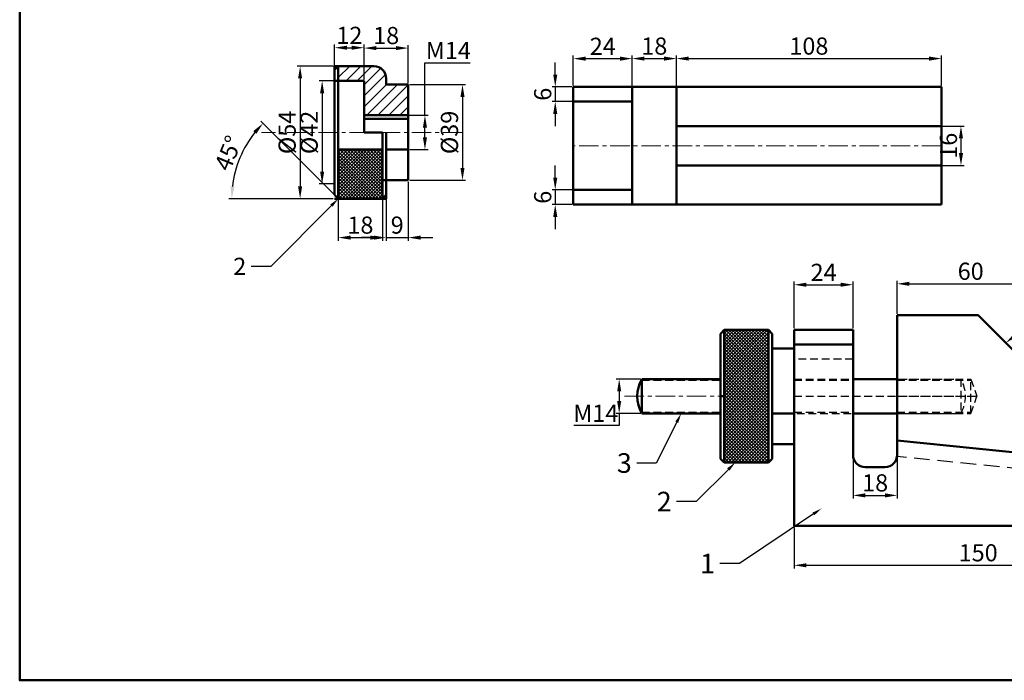
# Model space of a CAD drawing. Units: millimetres. Extents: x -238 to 500, y -191 to 322.
# Tile 1 of 3: x -238 to 164, y -152 to 117. Entities that reach past the tile are written whole.
import ezdxf
from ezdxf import colors
from ezdxf.entities.mleader import LeaderData, LeaderLine
from ezdxf.math import Vec2, Vec3

# ---------------------------------------------------------------- set-up
doc = ezdxf.new("R2010")
doc.units = ezdxf.units.MM
doc.header["$LTSCALE"] = 0.5
doc.linetypes.add('CENTER', pattern=[50.8, 31.75, -6.35, 6.35, -6.35])
doc.linetypes.add('DASHED', pattern=[19.05, 12.7, -6.35])
for name, color, linetype, lineweight in [('M-CNTR', 1, 'CENTER', 18), ('M-DIMS', 2, 'Continuous', 25), ('M-HATC', 8, 'Continuous', 18), ('M-HIDN', 6, 'DASHED', 25), ('M-OUTL', 7, 'Continuous', 50), ('M-TEXT', 3, 'Continuous', 25), ('M-TTLB', 7, 'Continuous', 50)]:
    doc.layers.add(name, color=color, linetype=linetype, lineweight=lineweight)
doc.styles.get("Standard").update_dxf_attribs({"font": 'arial.ttf'})
doc.dimstyles.new('ISO-25', dxfattribs={"dimtxt": 7, "dimasz": 5, "dimexe": 1.25, "dimexo": 0.625, "dimtad": 1, "dimtoh": 1, "dimtxsty": 'Standard', "dimcen": 2.5, "dimadec": 0, "dimazin": 0, "dimtfac": 1, "dimtmove": 0, "dimatfit": 3, "dimfxl": 1, "dimarcsym": 0})

# ---------------------------------------------------------------- blocks, each defined once
blk = doc.blocks.new('*D18')
at = {"layer": 'Defpoints', "color": 0, "ltscale": 0.5, "transparency": 16777216}
for p in [(11.98, 101.04), (-12.02, 89.53), (11.98, 89.53)]:
    blk.add_point(p, dxfattribs=at)
at = {"layer": 'M-DIMS', "color": 0, "lineweight": -2, "ltscale": 0.5, "transparency": 16777216}
for p, q in [((-12.02, 90.15), (-12.02, 102.29)), ((-7.02, 101.04), (6.98, 101.04)), ((11.98, 90.15), (11.98, 102.29))]:
    blk.add_line(p, q, dxfattribs=at)
at = {"layer": 'M-DIMS', "color": 0, "ltscale": 0.5, "transparency": 16777216}
for points in [[(-7.02, 101.87), (-7.02, 100.2), (-12.02, 101.04)], [(6.98, 101.87), (6.98, 100.2), (11.98, 101.04)]]:
    blk.add_solid(points, dxfattribs=at)
at = {"layer": 'M-DIMS', "color": 0, "ltscale": 0.5, "transparency": 16777216, "insert": (-0.02, 105.17), "char_height": 7, "attachment_point": 5}
blk.add_mtext('24', dxfattribs=at)
blk = doc.blocks.new('*D19')
at = {"layer": 'Defpoints', "color": 0, "ltscale": 0.5, "transparency": 16777216}
for p in [(29.98, 101.07), (11.98, 89.53), (29.98, 89.53)]:
    blk.add_point(p, dxfattribs=at)
at = {"layer": 'M-DIMS', "color": 0, "lineweight": -2, "ltscale": 0.5, "transparency": 16777216}
for p, q in [((11.98, 90.15), (11.98, 102.32)), ((16.98, 101.07), (24.98, 101.07)), ((29.98, 90.15), (29.98, 102.32))]:
    blk.add_line(p, q, dxfattribs=at)
at = {"layer": 'M-DIMS', "color": 0, "ltscale": 0.5, "transparency": 16777216}
for points in [[(16.98, 101.9), (16.98, 100.23), (11.98, 101.07)], [(24.98, 101.9), (24.98, 100.23), (29.98, 101.07)]]:
    blk.add_solid(points, dxfattribs=at)
at = {"layer": 'M-DIMS', "color": 0, "ltscale": 0.5, "transparency": 16777216, "insert": (20.98, 105.26), "char_height": 7, "attachment_point": 5}
blk.add_mtext('18', dxfattribs=at)
blk = doc.blocks.new('*D20')
at = {"layer": 'Defpoints', "color": 0, "ltscale": 0.5, "transparency": 16777216}
for p in [(137.98, 101.07), (29.98, 89.53), (137.98, 89.53)]:
    blk.add_point(p, dxfattribs=at)
at = {"layer": 'M-DIMS', "color": 0, "lineweight": -2, "ltscale": 0.5, "transparency": 16777216}
for p, q in [((29.98, 90.15), (29.98, 102.32)), ((34.98, 101.07), (132.98, 101.07)), ((137.98, 90.15), (137.98, 102.32))]:
    blk.add_line(p, q, dxfattribs=at)
at = {"layer": 'M-DIMS', "color": 0, "ltscale": 0.5, "transparency": 16777216}
for points in [[(34.98, 101.9), (34.98, 100.23), (29.98, 101.07)], [(132.98, 101.9), (132.98, 100.23), (137.98, 101.07)]]:
    blk.add_solid(points, dxfattribs=at)
at = {"layer": 'M-DIMS', "color": 0, "ltscale": 0.5, "transparency": 16777216, "insert": (83.98, 105.26), "char_height": 7, "attachment_point": 5}
blk.add_mtext('108', dxfattribs=at)
blk = doc.blocks.new('*D21')
at = {"layer": 'Defpoints', "color": 0, "ltscale": 0.5, "transparency": 16777216}
for p in [(-12.02, 89.53), (-19.39, 83.53), (-12.02, 83.53)]:
    blk.add_point(p, dxfattribs=at)
at = {"layer": 'M-DIMS', "color": 0, "lineweight": -2, "ltscale": 0.5, "transparency": 16777216}
for p, q in [((-19.39, 94.53), (-19.39, 99.53)), ((-12.65, 89.53), (-20.64, 89.53)), ((-19.39, 89.53), (-19.39, 83.53)), ((-12.65, 83.53), (-20.64, 83.53)), ((-19.39, 78.53), (-19.39, 73.53))]:
    blk.add_line(p, q, dxfattribs=at)
at = {"layer": 'M-DIMS', "color": 0, "ltscale": 0.5, "transparency": 16777216}
for points in [[(-20.22, 94.53), (-18.55, 94.53), (-19.39, 89.53)], [(-20.22, 78.53), (-18.55, 78.53), (-19.39, 83.53)]]:
    blk.add_solid(points, dxfattribs=at)
at = {"layer": 'M-DIMS', "color": 0, "ltscale": 0.5, "transparency": 16777216, "insert": (-23.59, 86.53), "char_height": 7, "attachment_point": 5, "rotation": 90}
blk.add_mtext('6', dxfattribs=at)
blk = doc.blocks.new('*D22')
at = {"layer": 'Defpoints', "color": 0, "ltscale": 0.5, "transparency": 16777216}
for p in [(-12.02, 47.53), (-19.39, 41.53), (-12.02, 41.53)]:
    blk.add_point(p, dxfattribs=at)
at = {"layer": 'M-DIMS', "color": 0, "lineweight": -2, "ltscale": 0.5, "transparency": 16777216}
for p, q in [((-19.39, 52.53), (-19.39, 57.53)), ((-12.65, 47.53), (-20.64, 47.53)), ((-19.39, 47.53), (-19.39, 41.53)), ((-12.65, 41.53), (-20.64, 41.53)), ((-19.39, 36.53), (-19.39, 31.53))]:
    blk.add_line(p, q, dxfattribs=at)
at = {"layer": 'M-DIMS', "color": 0, "ltscale": 0.5, "transparency": 16777216}
for points in [[(-20.22, 52.53), (-18.55, 52.53), (-19.39, 47.53)], [(-20.22, 36.53), (-18.55, 36.53), (-19.39, 41.53)]]:
    blk.add_solid(points, dxfattribs=at)
at = {"layer": 'M-DIMS', "color": 0, "ltscale": 0.5, "transparency": 16777216, "insert": (-23.59, 44.53), "char_height": 7, "attachment_point": 5, "rotation": 90}
blk.add_mtext('6', dxfattribs=at)
blk = doc.blocks.new('*D23')
at = {"layer": 'Defpoints', "color": 0, "ltscale": 0.5, "transparency": 16777216}
for p in [(137.98, 73.53), (137.98, 57.53), (145.96, 57.53)]:
    blk.add_point(p, dxfattribs=at)
at = {"layer": 'M-DIMS', "color": 0, "lineweight": -2, "ltscale": 0.5, "transparency": 16777216}
for p, q in [((138.6, 73.53), (147.21, 73.53)), ((145.96, 68.53), (145.96, 62.53)), ((138.6, 57.53), (147.21, 57.53))]:
    blk.add_line(p, q, dxfattribs=at)
at = {"layer": 'M-DIMS', "color": 0, "ltscale": 0.5, "transparency": 16777216}
for points in [[(145.12, 68.53), (146.79, 68.53), (145.96, 73.53)], [(145.12, 62.53), (146.79, 62.53), (145.96, 57.53)]]:
    blk.add_solid(points, dxfattribs=at)
at = {"layer": 'M-DIMS', "color": 0, "ltscale": 0.5, "transparency": 16777216, "insert": (141.76, 65.53), "char_height": 7, "attachment_point": 5, "rotation": 90}
blk.add_mtext('16', dxfattribs=at)
blk = doc.blocks.new('*D24')
at = {"layer": 'Defpoints', "color": 0, "ltscale": 0.5, "transparency": 16777216}
for p in [(-97.29, 105.49), (-109.29, 92.12), (-97.29, 91.96)]:
    blk.add_point(p, dxfattribs=at)
at = {"layer": 'M-DIMS', "color": 0, "lineweight": -2, "ltscale": 0.5, "transparency": 16777216}
for p, q in [((-109.29, 92.75), (-109.29, 106.74)), ((-104.29, 105.49), (-102.29, 105.49)), ((-97.29, 92.58), (-97.29, 106.74))]:
    blk.add_line(p, q, dxfattribs=at)
at = {"layer": 'M-DIMS', "color": 0, "ltscale": 0.5, "transparency": 16777216}
for points in [[(-104.29, 106.32), (-104.29, 104.66), (-109.29, 105.49)], [(-102.29, 106.32), (-102.29, 104.66), (-97.29, 105.49)]]:
    blk.add_solid(points, dxfattribs=at)
at = {"layer": 'M-DIMS', "color": 0, "ltscale": 0.5, "transparency": 16777216, "insert": (-103.29, 109.63), "char_height": 7, "attachment_point": 5}
blk.add_mtext('12', dxfattribs=at)
blk = doc.blocks.new('*D25')
at = {"layer": 'Defpoints', "color": 0, "ltscale": 0.5, "transparency": 16777216}
for p in [(-79.29, 105.35), (-97.29, 91.96), (-79.29, 90.46)]:
    blk.add_point(p, dxfattribs=at)
at = {"layer": 'M-DIMS', "color": 0, "lineweight": -2, "ltscale": 0.5, "transparency": 16777216}
for p, q in [((-97.29, 92.58), (-97.29, 106.6)), ((-92.29, 105.35), (-84.29, 105.35)), ((-79.29, 91.08), (-79.29, 106.6))]:
    blk.add_line(p, q, dxfattribs=at)
at = {"layer": 'M-DIMS', "color": 0, "ltscale": 0.5, "transparency": 16777216}
for points in [[(-92.29, 106.18), (-92.29, 104.52), (-97.29, 105.35)], [(-84.29, 106.18), (-84.29, 104.52), (-79.29, 105.35)]]:
    blk.add_solid(points, dxfattribs=at)
at = {"layer": 'M-DIMS', "color": 0, "ltscale": 0.5, "transparency": 16777216, "insert": (-88.29, 109.55), "char_height": 7, "attachment_point": 5}
blk.add_mtext('18', dxfattribs=at)
blk = doc.blocks.new('*D26')
at = {"layer": 'Defpoints', "color": 0, "ltscale": 0.5, "transparency": 16777216}
for p in [(-79.29, 90.46), (-79.29, 51.46), (-57.19, 51.46)]:
    blk.add_point(p, dxfattribs=at)
at = {"layer": 'M-DIMS', "color": 0, "lineweight": -2, "ltscale": 0.5, "transparency": 16777216}
for p, q in [((-78.67, 90.46), (-55.94, 90.46)), ((-57.19, 85.46), (-57.19, 56.46)), ((-78.67, 51.46), (-55.94, 51.46))]:
    blk.add_line(p, q, dxfattribs=at)
at = {"layer": 'M-DIMS', "color": 0, "ltscale": 0.5, "transparency": 16777216}
for points in [[(-58.02, 85.46), (-56.36, 85.46), (-57.19, 90.46)], [(-58.02, 56.46), (-56.36, 56.46), (-57.19, 51.46)]]:
    blk.add_solid(points, dxfattribs=at)
at = {"layer": 'M-DIMS', "color": 0, "ltscale": 0.5, "transparency": 16777216, "insert": (-61.59, 70.96), "char_height": 7, "attachment_point": 5, "rotation": 90}
blk.add_mtext('%%C39', dxfattribs=at)
blk = doc.blocks.new('*D27')
at = {"layer": 'Defpoints', "color": 0, "ltscale": 0.5, "transparency": 16777216}
for p in [(-79.43, 77.96), (-79.29, 63.96), (-72.49, 63.96)]:
    blk.add_point(p, dxfattribs=at)
at = {"layer": 'M-DIMS', "color": 0, "lineweight": -2, "ltscale": 0.5, "transparency": 16777216}
for p, q in [((-72.49, 77.96), (-72.49, 99.33)), ((-72.49, 99.33), (-54.04, 99.33)), ((-78.81, 77.96), (-71.24, 77.96)), ((-72.49, 68.96), (-72.49, 72.96)), ((-78.67, 63.96), (-71.24, 63.96))]:
    blk.add_line(p, q, dxfattribs=at)
at = {"layer": 'M-DIMS', "color": 0, "ltscale": 0.5, "transparency": 16777216}
for points in [[(-73.32, 72.96), (-71.66, 72.96), (-72.49, 77.96)], [(-73.32, 68.96), (-71.66, 68.96), (-72.49, 63.96)]]:
    blk.add_solid(points, dxfattribs=at)
at = {"layer": 'M-DIMS', "color": 0, "ltscale": 0.5, "transparency": 16777216, "insert": (-62.95, 103.47), "char_height": 7, "attachment_point": 5}
blk.add_mtext('M14', dxfattribs=at)
blk = doc.blocks.new('*D28')
at = {"layer": 'Defpoints', "color": 0, "ltscale": 0.5, "transparency": 16777216}
for p in [(-107.79, 43.96), (-89.79, 43.96), (-89.79, 28.08)]:
    blk.add_point(p, dxfattribs=at)
at = {"layer": 'M-DIMS', "color": 0, "lineweight": -2, "ltscale": 0.5, "transparency": 16777216}
for p, q in [((-107.79, 43.33), (-107.79, 26.83)), ((-89.79, 43.33), (-89.79, 26.83)), ((-102.79, 28.08), (-94.79, 28.08))]:
    blk.add_line(p, q, dxfattribs=at)
at = {"layer": 'M-DIMS', "color": 0, "ltscale": 0.5, "transparency": 16777216}
for points in [[(-102.79, 28.92), (-102.79, 27.25), (-107.79, 28.08)], [(-94.79, 28.92), (-94.79, 27.25), (-89.79, 28.08)]]:
    blk.add_solid(points, dxfattribs=at)
at = {"layer": 'M-DIMS', "color": 0, "ltscale": 0.5, "transparency": 16777216, "insert": (-98.79, 32.28), "char_height": 7, "attachment_point": 5}
blk.add_mtext('18', dxfattribs=at)
blk = doc.blocks.new('*D29')
at = {"layer": 'Defpoints', "color": 0, "ltscale": 0.5, "transparency": 16777216}
for p in [(-88.29, 49.96), (-79.29, 51.46), (-79.29, 28.08)]:
    blk.add_point(p, dxfattribs=at)
at = {"layer": 'M-DIMS', "color": 0, "lineweight": -2, "ltscale": 0.5, "transparency": 16777216}
for p, q in [((-88.29, 49.33), (-88.29, 26.83)), ((-79.29, 50.83), (-79.29, 26.83)), ((-93.29, 28.08), (-98.29, 28.08)), ((-88.29, 28.08), (-79.29, 28.08)), ((-74.29, 28.08), (-69.29, 28.08))]:
    blk.add_line(p, q, dxfattribs=at)
at = {"layer": 'M-DIMS', "color": 0, "ltscale": 0.5, "transparency": 16777216}
for points in [[(-93.29, 28.92), (-93.29, 27.25), (-88.29, 28.08)], [(-74.29, 28.92), (-74.29, 27.25), (-79.29, 28.08)]]:
    blk.add_solid(points, dxfattribs=at)
at = {"layer": 'M-DIMS', "color": 0, "ltscale": 0.5, "transparency": 16777216, "insert": (-83.79, 32.28), "char_height": 7, "attachment_point": 5}
blk.add_mtext('9', dxfattribs=at)
blk = doc.blocks.new('*D30')
at = {"layer": 'Defpoints', "color": 0, "ltscale": 0.5, "transparency": 16777216}
for p in [(-109.29, 91.96), (-114.39, 49.96), (-109.29, 49.96)]:
    blk.add_point(p, dxfattribs=at)
at = {"layer": 'M-DIMS', "color": 0, "lineweight": -2, "ltscale": 0.5, "transparency": 16777216}
for p, q in [((-109.92, 91.96), (-115.64, 91.96)), ((-114.39, 86.96), (-114.39, 54.96)), ((-109.92, 49.96), (-115.64, 49.96))]:
    blk.add_line(p, q, dxfattribs=at)
at = {"layer": 'M-DIMS', "color": 0, "ltscale": 0.5, "transparency": 16777216}
for points in [[(-115.22, 86.96), (-113.55, 86.96), (-114.39, 91.96)], [(-115.22, 54.96), (-113.55, 54.96), (-114.39, 49.96)]]:
    blk.add_solid(points, dxfattribs=at)
at = {"layer": 'M-DIMS', "color": 0, "ltscale": 0.5, "transparency": 16777216, "insert": (-118.78, 70.96), "char_height": 7, "attachment_point": 5, "rotation": 90}
blk.add_mtext('%%C42', dxfattribs=at)
blk = doc.blocks.new('*D31')
at = {"layer": 'Defpoints', "color": 0, "ltscale": 0.5, "transparency": 16777216}
for p in [(-109.29, 97.96), (-123.36, 43.96), (-109.29, 43.96)]:
    blk.add_point(p, dxfattribs=at)
at = {"layer": 'M-DIMS', "color": 0, "lineweight": -2, "ltscale": 0.5, "transparency": 16777216}
for p, q in [((-109.92, 97.96), (-124.61, 97.96)), ((-123.36, 92.96), (-123.36, 48.96)), ((-109.92, 43.96), (-124.61, 43.96))]:
    blk.add_line(p, q, dxfattribs=at)
at = {"layer": 'M-DIMS', "color": 0, "ltscale": 0.5, "transparency": 16777216}
for points in [[(-124.2, 92.96), (-122.53, 92.96), (-123.36, 97.96)], [(-124.2, 48.96), (-122.53, 48.96), (-123.36, 43.96)]]:
    blk.add_solid(points, dxfattribs=at)
at = {"layer": 'M-DIMS', "color": 0, "ltscale": 0.5, "transparency": 16777216, "insert": (-127.76, 70.96), "char_height": 7, "attachment_point": 5, "rotation": 90}
blk.add_mtext('%%C54', dxfattribs=at)
blk = doc.blocks.new('*D45')
at = {"layer": 'Defpoints', "color": 0, "ltscale": 0.5, "transparency": 16777216}
for p in [(-145.4, 65.67), (-109.29, 45.46), (-109.29, 43.96), (-107.79, 43.96), (-88.29, 43.96)]:
    blk.add_point(p, dxfattribs=at)
at = {"layer": 'M-DIMS', "color": 0, "lineweight": -2, "ltscale": 0.5, "transparency": 16777216}
for p, q in [((-109.73, 45.9), (-139.38, 75.55)), ((-109.92, 43.96), (-152.47, 43.96))]:
    blk.add_line(p, q, dxfattribs=at)
blk.add_arc((-107.79, 43.96), 43.43, 141.6, 173.4, dxfattribs=at)
at = {"layer": 'M-DIMS', "color": 0, "ltscale": 0.5, "transparency": 16777216}
for points in [[(-142.45, 71.49), (-141.2, 70.38), (-138.5, 74.67)], [(-150.1, 48.9), (-151.76, 49), (-151.22, 43.96)]]:
    blk.add_solid(points, dxfattribs=at)
at = {"layer": 'M-DIMS', "color": 0, "ltscale": 0.5, "transparency": 16777216, "insert": (-151.78, 62.18), "char_height": 7, "attachment_point": 5, "rotation": 67.5}
blk.add_mtext('45°', dxfattribs=at)
blk = doc.blocks.new('*D46')
at = {"layer": 'Defpoints', "color": 0, "ltscale": 0.5, "transparency": 16777216}
for p in [(15.92, -29.57), (6.67, -43.57), (15.92, -43.57)]:
    blk.add_point(p, dxfattribs=at)
at = {"layer": 'M-DIMS', "color": 0, "lineweight": -2, "ltscale": 0.5, "transparency": 16777216}
for p, q in [((15.29, -29.57), (5.42, -29.57)), ((6.67, -34.57), (6.67, -38.57)), ((15.29, -43.57), (5.42, -43.57)), ((6.67, -43.57), (6.67, -48.57)), ((6.67, -48.57), (-11.78, -48.57))]:
    blk.add_line(p, q, dxfattribs=at)
at = {"layer": 'M-DIMS', "color": 0, "ltscale": 0.5, "transparency": 16777216}
for points in [[(5.84, -34.57), (7.5, -34.57), (6.67, -29.57)], [(5.84, -38.57), (7.5, -38.57), (6.67, -43.57)]]:
    blk.add_solid(points, dxfattribs=at)
at = {"layer": 'M-DIMS', "color": 0, "ltscale": 0.5, "transparency": 16777216, "insert": (-2.87, -44.43), "char_height": 7, "attachment_point": 5}
blk.add_mtext('M14', dxfattribs=at)
blk = doc.blocks.new('*D47')
at = {"layer": 'Defpoints', "color": 0, "ltscale": 0.5, "transparency": 16777216}
for p in [(101.97, 8.88), (77.97, -9.46), (101.97, -9.46)]:
    blk.add_point(p, dxfattribs=at)
at = {"layer": 'M-DIMS', "color": 0, "lineweight": -2, "ltscale": 0.5, "transparency": 16777216}
for p, q in [((77.97, -8.84), (77.97, 10.13)), ((82.97, 8.88), (96.97, 8.88)), ((101.97, -8.84), (101.97, 10.13))]:
    blk.add_line(p, q, dxfattribs=at)
at = {"layer": 'M-DIMS', "color": 0, "ltscale": 0.5, "transparency": 16777216}
for points in [[(82.97, 9.71), (82.97, 8.04), (77.97, 8.88)], [(96.97, 9.71), (96.97, 8.04), (101.97, 8.88)]]:
    blk.add_solid(points, dxfattribs=at)
at = {"layer": 'M-DIMS', "color": 0, "ltscale": 0.5, "transparency": 16777216, "insert": (89.97, 13.02), "char_height": 7, "attachment_point": 5}
blk.add_mtext('24', dxfattribs=at)
blk = doc.blocks.new('*D48')
at = {"layer": 'Defpoints', "color": 0, "ltscale": 0.5, "transparency": 16777216}
for p in [(77.97, -89.46), (227.97, -89.46), (227.97, -105.49)]:
    blk.add_point(p, dxfattribs=at)
at = {"layer": 'M-DIMS', "color": 0, "lineweight": -2, "ltscale": 0.5, "transparency": 16777216}
for p, q in [((77.97, -90.09), (77.97, -106.74)), ((227.97, -90.09), (227.97, -106.74)), ((82.97, -105.49), (222.97, -105.49))]:
    blk.add_line(p, q, dxfattribs=at)
at = {"layer": 'M-DIMS', "color": 0, "ltscale": 0.5, "transparency": 16777216}
for points in [[(82.97, -104.66), (82.97, -106.32), (77.97, -105.49)], [(222.97, -104.66), (222.97, -106.32), (227.97, -105.49)]]:
    blk.add_solid(points, dxfattribs=at)
at = {"layer": 'M-DIMS', "color": 0, "ltscale": 0.5, "transparency": 16777216, "insert": (152.97, -101.29), "char_height": 7, "attachment_point": 5}
blk.add_mtext('150', dxfattribs=at)
blk = doc.blocks.new('*D49')
at = {"layer": 'Defpoints', "color": 0, "ltscale": 0.5, "transparency": 16777216}
for p in [(152.92, -3.57), (206.92, -3.57), (185.67, -9.09), (178.86, -29.51), (180.98, -29.51)]:
    blk.add_point(p, dxfattribs=at)
at = {"layer": 'M-DIMS', "color": 0, "lineweight": -2, "ltscale": 0.5, "transparency": 16777216}
blk.add_arc((179.92, -30.57), 22.24, 57.9107, 122.0893, dxfattribs=at)
at = {"layer": 'M-DIMS', "color": 0, "ltscale": 0.5, "transparency": 16777216}
for points in [[(168.62, -12.38), (167.58, -11.08), (164.19, -14.85)], [(192.25, -11.08), (191.21, -12.38), (195.64, -14.85)]]:
    blk.add_solid(points, dxfattribs=at)
at = {"layer": 'M-DIMS', "color": 0, "ltscale": 0.5, "transparency": 16777216, "insert": (179.92, -4.14), "char_height": 7, "attachment_point": 5}
blk.add_mtext('90°', dxfattribs=at)
blk = doc.blocks.new('*D50')
at = {"layer": 'Defpoints', "color": 0, "ltscale": 0.5, "transparency": 16777216}
for p in [(179.92, 9.26), (119.92, -3.57), (179.92, -30.57)]:
    blk.add_point(p, dxfattribs=at)
at = {"layer": 'M-DIMS', "color": 0, "lineweight": -2, "ltscale": 0.5, "transparency": 16777216}
for p, q in [((119.92, -2.95), (119.92, 10.51)), ((124.92, 9.26), (174.92, 9.26)), ((179.92, -29.95), (179.92, 10.51))]:
    blk.add_line(p, q, dxfattribs=at)
at = {"layer": 'M-DIMS', "color": 0, "ltscale": 0.5, "transparency": 16777216}
for points in [[(124.92, 10.09), (124.92, 8.42), (119.92, 9.26)], [(174.92, 10.09), (174.92, 8.42), (179.92, 9.26)]]:
    blk.add_solid(points, dxfattribs=at)
at = {"layer": 'M-DIMS', "color": 0, "ltscale": 0.5, "transparency": 16777216, "insert": (149.92, 13.46), "char_height": 7, "attachment_point": 5}
blk.add_mtext('60', dxfattribs=at)
blk = doc.blocks.new('*D52')
at = {"layer": 'Defpoints', "color": 0, "ltscale": 0.5, "transparency": 16777216}
for p in [(101.97, -57.93), (119.97, -57.57), (119.97, -76.99)]:
    blk.add_point(p, dxfattribs=at)
at = {"layer": 'M-DIMS', "color": 0, "lineweight": -2, "ltscale": 0.5, "transparency": 16777216}
for p, q in [((101.97, -58.55), (101.97, -78.24)), ((119.97, -58.19), (119.97, -78.24)), ((106.97, -76.99), (114.97, -76.99))]:
    blk.add_line(p, q, dxfattribs=at)
at = {"layer": 'M-DIMS', "color": 0, "ltscale": 0.5, "transparency": 16777216}
for points in [[(106.97, -76.16), (106.97, -77.83), (101.97, -76.99)], [(114.97, -76.16), (114.97, -77.83), (119.97, -76.99)]]:
    blk.add_solid(points, dxfattribs=at)
at = {"layer": 'M-DIMS', "color": 0, "ltscale": 0.5, "transparency": 16777216, "insert": (110.97, -72.8), "char_height": 7, "attachment_point": 5}
blk.add_mtext('18', dxfattribs=at)

msp = doc.modelspace()

# ---------------------------------------------------------------- hatches: boundary and pattern name
at = {"layer": 'M-HATC', "ltscale": 0.5}
h = msp.add_hatch(dxfattribs=at)
h.set_pattern_fill('ANSI31', color=256)
h.set_pattern_definition([(45, (-358.118, -179.4643), (-2.245064, 2.245064), [])])
h.paths.add_polyline_path([(-97.291, 77.958), (-79.291, 77.958), (-79.291, 90.458), (-88.291, 90.458), (-88.291, 92.958, 0.4142136), (-93.291, 97.958), (-107.791, 97.958), (-107.791, 91.958), (-97.291, 91.958)])
h = msp.add_hatch(dxfattribs=at)
h.set_pattern_fill('ANSI37', color=256, scale=0.3)
h.set_pattern_definition([(45, (-358.1179, -179.4643), (-0.6735192, 0.6735192), []), (135, (-358.1179, -179.4643), (-0.6735192, -0.6735192), [])])
h.paths.add_polyline_path([(-107.791, 43.958), (-89.791, 43.958), (-89.791, 63.958), (-107.791, 63.958)])
h = msp.add_hatch(dxfattribs=at)
h.set_pattern_fill('ANSI37', color=256, scale=0.3)
h.set_pattern_definition([(45, (-1017.7025, -621.6411), (-0.6735192, 0.6735192), []), (135, (-1017.7025, -621.6411), (-0.6735192, -0.6735192), [])])
h.paths.add_polyline_path([(67.469, -17.072), (67.469, -9.572), (49.469, -9.572), (49.469, -63.572), (67.469, -63.572)])

# ---------------------------------------------------------------- linework, layer by layer
at = {"layer": 'M-CNTR', "ltscale": 0.5}
for p, q in [((-57.191, 70.958), (-139.151, 70.958)), ((137.976, 65.529), (-12.024, 65.529)), ((8.799, -36.572), (49.469, -36.572))]:
    msp.add_line(p, q, dxfattribs=at)
at = {"layer": 'M-HIDN', "ltscale": 0.5}
for p, q in [((101.969, -21.465), (77.969, -21.465)), ((15.916, -30.072), (47.969, -30.072)), ((77.969, -29.572), (145.916, -29.572)), ((77.969, -30.072), (101.969, -30.072)), ((119.916, -29.572), (149.916, -29.572)), ((119.916, -30.072), (145.916, -30.072)), ((119.916, -30.072), (149.916, -30.072)), ((145.916, -29.572), (145.916, -43.572)), ((149.916, -43.572), (149.916, -29.572)), ((149.916, -29.572), (152.464, -36.572)), ((77.969, -36.572), (153.69, -36.572)), ((119.916, -36.572), (149.916, -36.572)), ((149.916, -43.572), (152.464, -36.572)), ((15.916, -43.072), (47.969, -43.072)), ((69.517, -43.572), (145.916, -43.572)), ((77.969, -43.072), (101.969, -43.072)), ((119.916, -43.072), (145.916, -43.072)), ((119.916, -43.072), (149.916, -43.072)), ((119.916, -43.572), (149.916, -43.572))]:
    msp.add_line(p, q, dxfattribs=at)
at = {"layer": 'M-HIDN'}
msp.add_line((227.969, -71.997), (119.916, -61.193), dxfattribs=at)
at = {"layer": 'M-HIDN', "ltscale": 0.5}
msp.add_arc((133.791, -36.572), 14, 330, 30, dxfattribs=at)
at = {"layer": 'M-OUTL', "ltscale": 0.5}
for p, q in [((-109.291, 97.958), (-109.291, 45.458)), ((-109.291, 97.958), (-93.291, 97.958)), ((-107.791, 97.958), (-109.291, 96.458)), ((-107.791, 97.958), (-107.791, 43.958)), ((-88.291, 92.958), (-88.291, 90.458)), ((-109.291, 91.958), (-97.291, 91.958)), ((-97.291, 91.958), (-97.291, 70.958)), ((-88.291, 90.458), (-79.291, 90.458)), ((-79.291, 90.458), (-79.291, 51.458)), ((-12.024, 89.529), (-12.024, 41.529)), ((11.976, 89.529), (-12.024, 89.529)), ((137.976, 89.529), (11.976, 89.529)), ((11.976, 89.529), (11.976, 41.529)), ((29.976, 89.529), (29.976, 41.529)), ((137.976, 41.529), (137.976, 89.529)), ((11.976, 83.529), (-12.024, 83.529)), ((-79.431, 77.958), (-97.291, 77.958)), ((-79.291, 76.458), (-97.291, 76.458)), ((-79.291, 77.958), (-95.791, 77.958)), ((137.976, 73.529), (29.976, 73.529)), ((-97.291, 70.958), (-89.791, 70.958)), ((-89.791, 43.958), (-89.791, 70.958)), ((-88.291, 43.958), (-88.291, 70.958)), ((-89.791, 63.958), (-107.791, 63.958)), ((-79.291, 63.958), (-88.291, 63.958)), ((137.976, 57.529), (29.976, 57.529)), ((-79.291, 51.458), (-89.791, 51.458)), ((-107.791, 43.958), (-109.291, 45.458)), ((-89.791, 43.958), (-88.291, 45.458)), ((-12.024, 47.529), (11.976, 47.529)), ((-109.291, 43.958), (-88.291, 43.958)), ((-12.024, 41.529), (11.976, 41.529)), ((11.976, 41.529), (137.976, 41.529)), ((119.916, -3.572), (152.916, -3.572)), ((119.916, -3.572), (119.916, -36.572)), ((178.855, -29.511), (152.916, -3.572)), ((49.469, -9.572), (47.969, -11.072)), ((47.969, -11.072), (47.969, -62.072)), ((49.469, -9.572), (67.469, -9.572)), ((49.469, -9.572), (49.469, -63.572)), ((67.469, -17.072), (67.469, -9.572)), ((67.469, -9.572), (68.969, -11.072)), ((68.969, -11.072), (68.969, -17.072)), ((67.469, -63.572), (67.469, -17.072)), ((68.969, -17.072), (77.969, -17.072)), ((68.969, -62.072), (68.969, -17.072)), ((77.969, -17.072), (77.969, -56.072)), ((15.916, -29.572), (47.969, -29.572)), ((15.916, -29.572), (15.916, -43.572)), ((101.969, -29.572), (120.416, -29.572)), ((119.916, -29.572), (119.916, -43.572)), ((49.469, -36.572), (47.969, -36.572)), ((119.916, -36.572), (119.916, -61.193)), ((15.916, -43.572), (47.969, -43.572)), ((77.969, -43.572), (68.969, -43.572)), ((101.969, -43.572), (119.916, -43.572)), ((77.969, -56.072), (68.969, -56.072)), ((233.916, -66.039), (119.916, -54.661)), ((49.469, -63.572), (47.969, -62.072)), ((49.469, -63.572), (67.469, -63.572)), ((67.469, -63.572), (68.969, -62.072))]:
    msp.add_line(p, q, dxfattribs=at)
at = {"layer": 'M-OUTL'}
for p, q in [((77.969, -9.465), (77.969, -89.465)), ((77.969, -9.465), (101.969, -9.465)), ((101.969, -9.465), (101.969, -60.465)), ((77.969, -15.465), (101.969, -15.465)), ((227.969, -65.465), (119.969, -54.666)), ((119.969, -54.666), (119.969, -60.465)), ((106.969, -65.465), (114.969, -65.465)), ((77.969, -89.465), (227.969, -89.465))]:
    msp.add_line(p, q, dxfattribs=at)
at = {"layer": 'M-OUTL', "ltscale": 0.5}
for centre, radius, start, end in [((-93.291, 92.958), 5, 0, 90), ((28.04, -36.572), 14, 150, 210)]:
    msp.add_arc(centre, radius, start, end, dxfattribs=at)
at = {"layer": 'M-OUTL'}
for centre, start, end in [((106.969, -60.465), 180, 270), ((114.969, -60.465), 270, 0)]:
    msp.add_arc(centre, 5, start, end, dxfattribs=at)
at = {"layer": 'M-TTLB', "ltscale": 0.5}
msp.add_lwpolyline([(-237.643, 321.636), (499.641, 321.636), (499.641, -152.379), (-237.643, -152.379)], close=True, dxfattribs=at)

# ---------------------------------------------------------------- dimensions: what is measured, and where the dimension line sits
at = {"layer": 'M-DIMS', "ltscale": 0.5}
for base, p1, p2, picture, middle in [((-97.291, 105.491), (-109.291, 92.125), (-97.291, 91.958), '*D24', (-103.291, 109.631)), ((-79.291, 105.349), (-97.291, 91.958), (-79.291, 90.458), '*D25', (-88.291, 109.548)), ((11.976, 101.035), (-12.024, 89.529), (11.976, 89.529), '*D18', (-0.024, 105.174)), ((29.976, 101.065), (11.976, 89.529), (29.976, 89.529), '*D19', (20.976, 105.264)), ((137.976, 101.065), (29.976, 89.529), (137.976, 89.529), '*D20', (83.976, 105.264)), ((-79.291, 28.083), (-88.291, 49.958), (-79.291, 51.458), '*D29', (-83.791, 32.282)), ((101.969, 8.878), (77.969, -9.465), (101.969, -9.465), '*D47', (89.969, 13.017)), ((179.916, 9.257), (119.916, -3.572), (179.916, -30.572), '*D50', (149.916, 13.456)), ((119.969, -76.994), (101.969, -57.926), (119.969, -57.565), '*D52', (110.969, -72.795)), ((227.969, -105.49), (77.969, -89.465), (227.969, -89.465), '*D48', (152.969, -101.291))]:
    dim = msp.add_linear_dim(base=base, p1=p1, p2=p2, dimstyle='ISO-25', override={"dimclrd": 0, "dimclre": 0, "dimclrt": 0}, dxfattribs=at)
    dim.commit()
    dim.dimension.update_dxf_attribs({"geometry": picture, "text_midpoint": middle})
for base, p1, p2, text, picture, middle in [((-72.491, 63.958), (-79.431, 77.958), (-79.291, 63.958), 'M<>', '*D27', (-62.954, 99.331)), ((-57.191, 51.458), (-79.291, 90.458), (-79.291, 51.458), '%%C<>', '*D26', (-57.191, 70.958))]:
    dim = msp.add_linear_dim(base=base, p1=p1, p2=p2, angle=90, text=text, dimstyle='ISO-25', override={"dimclrd": 0, "dimclre": 0, "dimclrt": 0}, dxfattribs=at)
    dim.commit()
    dim.dimension.update_dxf_attribs({"geometry": picture, "text_midpoint": middle, "dimtype": 160})
for base, p1, p2, text, picture, middle in [((-123.363, 43.958), (-109.291, 97.958), (-109.291, 43.958), '%%C<>', '*D31', (-127.757, 70.958)), ((-114.386, 49.958), (-109.291, 91.958), (-109.291, 49.958), '%%C<>', '*D30', (-118.78, 70.958)), ((6.671, -43.572), (15.916, -29.572), (15.916, -43.572), 'M<>', '*D46', (-2.867, -44.432))]:
    dim = msp.add_linear_dim(base=base, p1=p1, p2=p2, angle=90, text=text, dimstyle='ISO-25', override={"dimclrd": 0, "dimclre": 0, "dimclrt": 0}, dxfattribs=at)
    dim.commit()
    dim.dimension.update_dxf_attribs({"geometry": picture, "text_midpoint": middle})
for base, p1, p2, picture, middle in [((-19.387, 83.529), (-12.024, 89.529), (-12.024, 83.529), '*D21', (-23.586, 86.529)), ((145.956, 57.529), (137.976, 73.529), (137.976, 57.529), '*D23', (141.757, 65.529)), ((-19.387, 41.529), (-12.024, 47.529), (-12.024, 41.529), '*D22', (-23.586, 44.529))]:
    dim = msp.add_linear_dim(base=base, p1=p1, p2=p2, angle=90, dimstyle='ISO-25', override={"dimclrd": 0, "dimclre": 0, "dimclrt": 0}, dxfattribs=at)
    dim.commit()
    dim.dimension.update_dxf_attribs({"geometry": picture, "text_midpoint": middle})
for base, line1, line2, picture, middle in [((-145.402, 65.673), ((-109.291, 43.958), (-88.291, 43.958)), ((-107.791, 43.958), (-109.291, 45.458)), '*D45', (-151.781, 62.179)), ((185.671, -9.093), ((180.976, -29.511), (206.916, -3.572)), ((178.855, -29.511), (152.916, -3.572)), '*D49', (179.916, -4.136))]:
    dim = msp.add_angular_dim_2l(base=base, line1=line1, line2=line2, dimstyle='ISO-25', override={"dimclrd": 0, "dimclre": 0, "dimclrt": 0}, dxfattribs=at)
    dim.commit()
    dim.dimension.update_dxf_attribs({"geometry": picture, "text_midpoint": middle})
dim = msp.add_linear_dim(base=(-89.791, 28.083), p1=(-107.791, 43.958), p2=(-89.791, 43.958), dimstyle='ISO-25', override={"dimclrd": 0, "dimclre": 0, "dimclrt": 0}, dxfattribs=at)
dim.commit()
dim.dimension.update_dxf_attribs({"geometry": '*D28', "text_midpoint": (-98.791, 28.083), "dimtype": 160})

# ---------------------------------------------------------------- leaders
at = {"layer": 'M-TEXT', "ltscale": 0.5}
ml = msp.add_multileader_mtext('Standard', dxfattribs=at)
ml.set_content('2', color=256)
ml.set_leader_properties()
ml.build(insert=Vec2(0, 0))
ctx = ml.context
ctx.base_point, ctx.char_height, ctx.plane_origin = Vec3(-151.96, 16.368), 7, Vec3(-107.791, 43.958)
ctx.text_align_type = 2
notes = []
notes.append((ctx, [(0, (1, 1, 0), (-135.323, 16.368), (-1, 0), 8, [(0, [(-107.791, 43.958)], 0, [])])]))
ctx.mtext.insert, ctx.mtext.alignment, ctx.mtext.flow_direction = Vec3(-145.323, 19.868), 3, 5
ml = msp.add_multileader_mtext('Standard', dxfattribs=at)
ml.set_content('3', color=256)
ml.set_leader_properties()
ml.build(insert=Vec2(0, 0))
ctx = ml.context
ctx.base_point, ctx.char_height, ctx.plane_origin = Vec3(4.561, -63.87), 8, Vec3(31.942, -43.572)
ctx.text_align_type = 2
notes.append((ctx, [(0, (1, 1, 0), (21.8, -63.87), (-1, 0), 8, [(0, [(31.942, -43.572)], 0, [])])]))
ctx.mtext.insert, ctx.mtext.alignment, ctx.mtext.flow_direction = Vec3(11.8, -59.799), 3, 5
ml = msp.add_multileader_mtext('Standard', dxfattribs=at)
ml.set_content('2', color=256)
ml.set_leader_properties()
ml.build(insert=Vec2(0, 0))
ctx = ml.context
ctx.base_point, ctx.char_height, ctx.plane_origin = Vec3(20.744, -79.528), 8, Vec3(53.999, -63.572)
ctx.text_align_type = 2
notes.append((ctx, [(0, (1, 1, 0), (38.043, -79.528), (-1, 0), 8, [(0, [(53.999, -63.572)], 0, [])])]))
ctx.mtext.insert, ctx.mtext.alignment, ctx.mtext.flow_direction = Vec3(28.043, -75.528), 3, 5
ml = msp.add_multileader_mtext('Standard', dxfattribs=at)
ml.set_content('1', color=256)
ml.set_leader_properties()
ml.build(insert=Vec2(0, 0))
ctx = ml.context
ctx.base_point, ctx.char_height, ctx.plane_origin = Vec3(40.741, -104.776), 8, Vec3(89.147, -82.327)
ctx.text_align_type = 2
notes.append((ctx, [(0, (1, 1, 0), (55.687, -104.776), (-1, 0), 8, [(0, [(89.147, -82.327)], 0, [])])]))
ctx.mtext.insert, ctx.mtext.alignment, ctx.mtext.flow_direction = Vec3(45.687, -100.776), 3, 5
for ctx, leaders in notes:
    for number, flags, end, landing, length, lines in leaders:
        leader = LeaderData()
        leader.index, (leader.has_last_leader_line, leader.has_dogleg_vector, leader.attachment_direction) = number, flags
        leader.last_leader_point, leader.dogleg_vector, leader.dogleg_length = Vec3(end), Vec3(landing), length
        for number, points, colour, breaks in lines:
            line = LeaderLine()
            line.index, line.vertices, line.color, line.breaks = number, Vec3.list(points), colors.encode_raw_color(colour), breaks
            leader.lines.append(line)
        ctx.leaders.append(leader)

doc.saveas('drawing.dxf')
